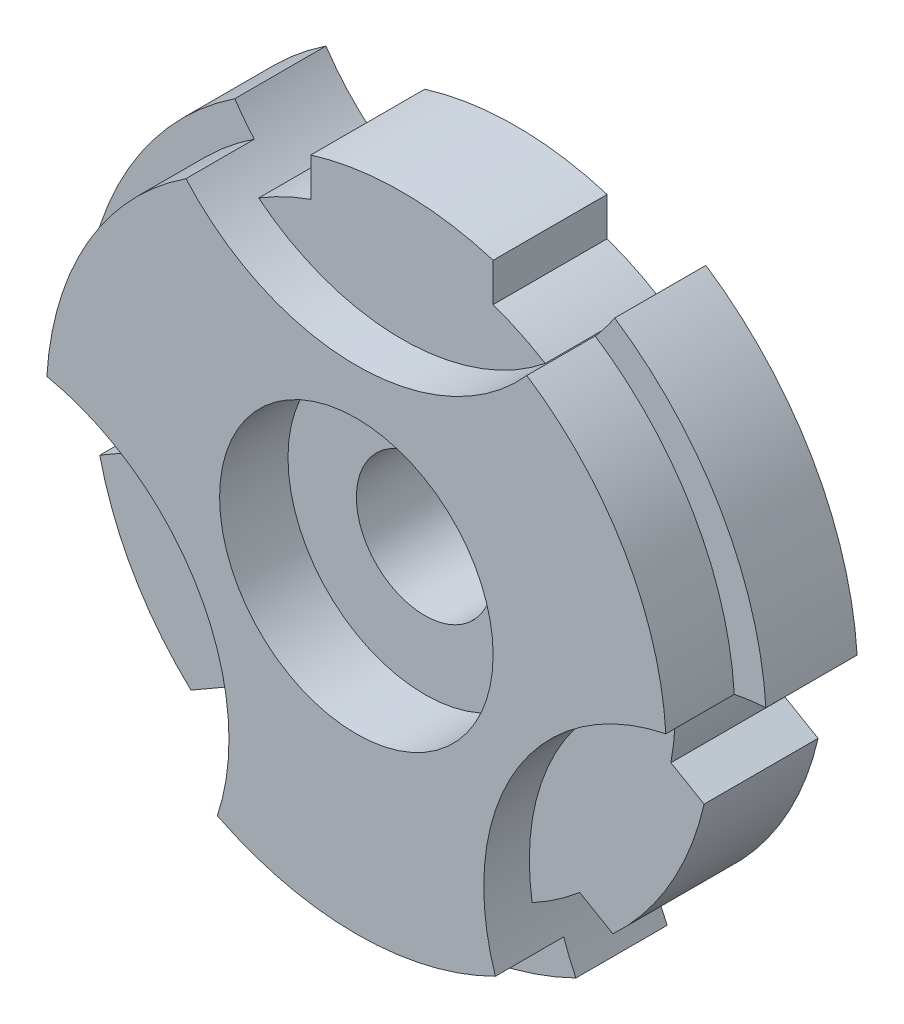
ISO-10303-21;
HEADER;
FILE_DESCRIPTION(('STEP AP214'),'2;1');
FILE_NAME('part.step','',(''),(''),'','','');
FILE_SCHEMA(('AUTOMOTIVE_DESIGN { 1 0 10303 214 1 1 1 1 }'));
ENDSEC;
DATA;
#1=APPLICATION_CONTEXT('core data for automotive mechanical design processes');
#2=APPLICATION_PROTOCOL_DEFINITION('international standard','automotive_design',2000,#1);
#3=PRODUCT_CONTEXT('',#1,'mechanical');
#4=PRODUCT('Part','Part','',(#3));
#5=PRODUCT_RELATED_PRODUCT_CATEGORY('part','',(#4));
#6=PRODUCT_DEFINITION_FORMATION('','',#4);
#7=PRODUCT_DEFINITION_CONTEXT('part definition',#1,'design');
#8=PRODUCT_DEFINITION('design','',#6,#7);
#9=PRODUCT_DEFINITION_SHAPE('','',#8);
#10=(LENGTH_UNIT() NAMED_UNIT(*) SI_UNIT(.MILLI.,.METRE.));
#11=(NAMED_UNIT(*) PLANE_ANGLE_UNIT() SI_UNIT($,.RADIAN.));
#12=(NAMED_UNIT(*) SI_UNIT($,.STERADIAN.) SOLID_ANGLE_UNIT());
#13=UNCERTAINTY_MEASURE_WITH_UNIT(LENGTH_MEASURE(1.E-05),#10,'distance_accuracy_value','');
#14=(GEOMETRIC_REPRESENTATION_CONTEXT(3) GLOBAL_UNCERTAINTY_ASSIGNED_CONTEXT((#13)) GLOBAL_UNIT_ASSIGNED_CONTEXT((#10,
#11,#12)) REPRESENTATION_CONTEXT('',''));
#15=CARTESIAN_POINT('',(0.,0.,0.));
#16=DIRECTION('',(0.,0.,1.));
#17=DIRECTION('',(1.,0.,0.));
#18=AXIS2_PLACEMENT_3D('',#15,#16,#17);
#19=CARTESIAN_POINT('',(0.,0.,20.));
#20=DIRECTION('',(0.,0.,-1.));
#21=DIRECTION('',(-1.,0.,0.));
#22=AXIS2_PLACEMENT_3D('',#19,#20,#21);
#23=CYLINDRICAL_SURFACE('',#22,75.);
#24=CARTESIAN_POINT('',(0.,0.,0.));
#25=DIRECTION('',(0.,0.,1.));
#26=DIRECTION('',(1.,0.,0.));
#27=AXIS2_PLACEMENT_3D('',#24,#25,#26);
#28=CIRCLE('',#27,75.);
#29=CARTESIAN_POINT('',(74.8395240227173,4.90363579939592,0.));
#30=VERTEX_POINT('',#29);
#31=CARTESIAN_POINT('',(41.6664351845422,62.3611111111111,0.));
#32=VERTEX_POINT('',#31);
#33=EDGE_CURVE('E459',#30,#32,#28,.T.);
#34=ORIENTED_EDGE('',*,*,#33,.T.);
#35=DIRECTION('',(0.,0.,1.));
#36=VECTOR('',#35,1.);
#37=CARTESIAN_POINT('',(41.6664351845422,62.3611111111111,17.5));
#38=LINE('',#37,#36);
#39=CARTESIAN_POINT('',(41.6664351845422,62.3611111111111,20.));
#40=VERTEX_POINT('',#39);
#41=EDGE_CURVE('E438',#32,#40,#38,.T.);
#42=ORIENTED_EDGE('',*,*,#41,.T.);
#43=CARTESIAN_POINT('',(0.,0.,20.));
#44=DIRECTION('',(0.,0.,1.));
#45=DIRECTION('',(1.,0.,0.));
#46=AXIS2_PLACEMENT_3D('',#43,#44,#45);
#47=CIRCLE('',#46,75.);
#48=CARTESIAN_POINT('',(74.8395240227173,4.90363579939591,20.));
#49=VERTEX_POINT('',#48);
#50=EDGE_CURVE('E455',#49,#40,#47,.T.);
#51=ORIENTED_EDGE('',*,*,#50,.F.);
#52=DIRECTION('',(0.,0.,1.));
#53=VECTOR('',#52,1.);
#54=CARTESIAN_POINT('',(74.8395240227173,4.90363579939593,17.5));
#55=LINE('',#54,#53);
#56=EDGE_CURVE('E417',#49,#30,#55,.F.);
#57=ORIENTED_EDGE('',*,*,#56,.T.);
#58=EDGE_LOOP('',(#34,#42,#51,#57));
#59=FACE_BOUND('',#58,.T.);
#60=ADVANCED_FACE('F50',(#59),#23,.T.);
#61=CARTESIAN_POINT('',(-33.1730888381753,-67.2647469105068,0.));
#62=VERTEX_POINT('',#61);
#63=CARTESIAN_POINT('',(33.1730888381754,-67.2647469105067,0.));
#64=VERTEX_POINT('',#63);
#65=EDGE_CURVE('E446',#62,#64,#28,.T.);
#66=ORIENTED_EDGE('',*,*,#65,.T.);
#67=DIRECTION('',(0.,0.,1.));
#68=VECTOR('',#67,1.);
#69=CARTESIAN_POINT('',(33.1730888381754,-67.2647469105067,17.5));
#70=LINE('',#69,#68);
#71=CARTESIAN_POINT('',(33.1730888381754,-67.2647469105067,20.));
#72=VERTEX_POINT('',#71);
#73=EDGE_CURVE('E424',#64,#72,#70,.T.);
#74=ORIENTED_EDGE('',*,*,#73,.T.);
#75=CARTESIAN_POINT('',(-33.1730888381753,-67.2647469105068,20.));
#76=VERTEX_POINT('',#75);
#77=EDGE_CURVE('E456',#76,#72,#47,.T.);
#78=ORIENTED_EDGE('',*,*,#77,.F.);
#79=DIRECTION('',(0.,0.,1.));
#80=VECTOR('',#79,1.);
#81=CARTESIAN_POINT('',(-33.1730888381753,-67.2647469105068,17.5));
#82=LINE('',#81,#80);
#83=EDGE_CURVE('E405',#76,#62,#82,.F.);
#84=ORIENTED_EDGE('',*,*,#83,.T.);
#85=EDGE_LOOP('',(#66,#74,#78,#84));
#86=FACE_BOUND('',#85,.T.);
#87=ADVANCED_FACE('F498',(#86),#23,.T.);
#88=CARTESIAN_POINT('',(0.,0.,20.));
#89=DIRECTION('',(0.,0.,1.));
#90=DIRECTION('',(1.,0.,0.));
#91=AXIS2_PLACEMENT_3D('',#88,#89,#90);
#92=PLANE('',#91);
#93=CARTESIAN_POINT('',(0.,90.,20.));
#94=DIRECTION('',(0.,0.,1.));
#95=DIRECTION('',(1.,0.,0.));
#96=AXIS2_PLACEMENT_3D('',#93,#94,#95);
#97=CIRCLE('',#96,50.);
#98=CARTESIAN_POINT('',(-41.6664351845422,62.3611111111111,20.));
#99=VERTEX_POINT('',#98);
#100=CARTESIAN_POINT('',(-37.3866286257534,56.8,20.));
#101=VERTEX_POINT('',#100);
#102=EDGE_CURVE('E429',#99,#101,#97,.T.);
#103=ORIENTED_EDGE('',*,*,#102,.F.);
#104=CARTESIAN_POINT('',(-74.8395240227173,4.90363579939591,20.));
#105=VERTEX_POINT('',#104);
#106=EDGE_CURVE('E460',#99,#105,#47,.T.);
#107=ORIENTED_EDGE('',*,*,#106,.T.);
#108=CARTESIAN_POINT('',(-77.9422863405996,-44.9999999999998,20.));
#109=DIRECTION('',(0.,0.,1.));
#110=DIRECTION('',(1.,0.,0.));
#111=AXIS2_PLACEMENT_3D('',#108,#109,#110);
#112=CIRCLE('',#111,50.);
#113=CARTESIAN_POINT('',(-67.8835572478328,3.97777015175706,20.));
#114=VERTEX_POINT('',#113);
#115=EDGE_CURVE('E401',#114,#105,#112,.T.);
#116=ORIENTED_EDGE('',*,*,#115,.F.);
#117=CARTESIAN_POINT('',(0.,0.,20.));
#118=DIRECTION('',(0.,0.,1.));
#119=DIRECTION('',(1.,0.,0.));
#120=AXIS2_PLACEMENT_3D('',#117,#118,#119);
#121=CIRCLE('',#120,68.);
#122=EDGE_CURVE('E454',#101,#114,#121,.T.);
#123=ORIENTED_EDGE('',*,*,#122,.F.);
#124=EDGE_LOOP('',(#103,#107,#116,#123));
#125=FACE_BOUND('',#124,.T.);
#126=ADVANCED_FACE('F489',(#125),#92,.T.);
#127=CARTESIAN_POINT('',(37.3866286257534,56.8,20.));
#128=VERTEX_POINT('',#127);
#129=EDGE_CURVE('E433',#128,#40,#97,.T.);
#130=ORIENTED_EDGE('',*,*,#129,.F.);
#131=CARTESIAN_POINT('',(67.8835572478328,3.97777015175707,20.));
#132=VERTEX_POINT('',#131);
#133=EDGE_CURVE('E449',#132,#128,#121,.T.);
#134=ORIENTED_EDGE('',*,*,#133,.F.);
#135=CARTESIAN_POINT('',(77.9422863405996,-44.9999999999998,20.));
#136=DIRECTION('',(0.,0.,1.));
#137=DIRECTION('',(1.,0.,0.));
#138=AXIS2_PLACEMENT_3D('',#135,#136,#137);
#139=CIRCLE('',#138,50.);
#140=EDGE_CURVE('E411',#49,#132,#139,.T.);
#141=ORIENTED_EDGE('',*,*,#140,.F.);
#142=ORIENTED_EDGE('',*,*,#50,.T.);
#143=EDGE_LOOP('',(#130,#134,#141,#142));
#144=FACE_BOUND('',#143,.T.);
#145=ADVANCED_FACE('F542',(#144),#92,.T.);
#146=CARTESIAN_POINT('',(0.,0.,35.));
#147=DIRECTION('',(0.,0.,-1.));
#148=DIRECTION('',(-1.,0.,0.));
#149=AXIS2_PLACEMENT_3D('',#146,#147,#148);
#150=CYLINDRICAL_SURFACE('',#149,68.);
#151=ORIENTED_EDGE('',*,*,#133,.T.);
#152=DIRECTION('',(0.,0.,1.));
#153=VECTOR('',#152,1.);
#154=CARTESIAN_POINT('',(37.3866286257534,56.8,17.5));
#155=LINE('',#154,#153);
#156=CARTESIAN_POINT('',(37.3866286257534,56.8,35.));
#157=VERTEX_POINT('',#156);
#158=EDGE_CURVE('E436',#128,#157,#155,.T.);
#159=ORIENTED_EDGE('',*,*,#158,.T.);
#160=CARTESIAN_POINT('',(0.,0.,35.));
#161=DIRECTION('',(0.,0.,1.));
#162=DIRECTION('',(1.,0.,0.));
#163=AXIS2_PLACEMENT_3D('',#160,#161,#162);
#164=CIRCLE('',#163,68.);
#165=CARTESIAN_POINT('',(67.8835572478328,3.97777015175707,35.));
#166=VERTEX_POINT('',#165);
#167=EDGE_CURVE('E444',#166,#157,#164,.T.);
#168=ORIENTED_EDGE('',*,*,#167,.F.);
#169=DIRECTION('',(0.,0.,1.));
#170=VECTOR('',#169,1.);
#171=CARTESIAN_POINT('',(67.8835572478328,3.97777015175708,17.5));
#172=LINE('',#171,#170);
#173=EDGE_CURVE('E414',#166,#132,#172,.F.);
#174=ORIENTED_EDGE('',*,*,#173,.T.);
#175=EDGE_LOOP('',(#151,#159,#168,#174));
#176=FACE_BOUND('',#175,.T.);
#177=ADVANCED_FACE('F546',(#176),#150,.T.);
#178=CARTESIAN_POINT('',(-30.4969286220795,-60.7777701517569,20.));
#179=VERTEX_POINT('',#178);
#180=CARTESIAN_POINT('',(30.4969286220796,-60.7777701517568,20.));
#181=VERTEX_POINT('',#180);
#182=EDGE_CURVE('E452',#179,#181,#121,.T.);
#183=ORIENTED_EDGE('',*,*,#182,.T.);
#184=DIRECTION('',(0.,0.,1.));
#185=VECTOR('',#184,1.);
#186=CARTESIAN_POINT('',(30.4969286220796,-60.7777701517568,17.5));
#187=LINE('',#186,#185);
#188=CARTESIAN_POINT('',(30.4969286220796,-60.7777701517568,35.));
#189=VERTEX_POINT('',#188);
#190=EDGE_CURVE('E423',#181,#189,#187,.T.);
#191=ORIENTED_EDGE('',*,*,#190,.T.);
#192=CARTESIAN_POINT('',(-30.4969286220796,-60.7777701517568,35.));
#193=VERTEX_POINT('',#192);
#194=EDGE_CURVE('E445',#193,#189,#164,.T.);
#195=ORIENTED_EDGE('',*,*,#194,.F.);
#196=DIRECTION('',(0.,0.,1.));
#197=VECTOR('',#196,1.);
#198=CARTESIAN_POINT('',(-30.4969286220796,-60.7777701517568,17.5));
#199=LINE('',#198,#197);
#200=EDGE_CURVE('E388',#193,#179,#199,.F.);
#201=ORIENTED_EDGE('',*,*,#200,.T.);
#202=EDGE_LOOP('',(#183,#191,#195,#201));
#203=FACE_BOUND('',#202,.T.);
#204=ADVANCED_FACE('F475',(#203),#150,.T.);
#205=ORIENTED_EDGE('',*,*,#106,.F.);
#206=DIRECTION('',(0.,0.,1.));
#207=VECTOR('',#206,1.);
#208=CARTESIAN_POINT('',(-41.6664351845422,62.3611111111111,17.5));
#209=LINE('',#208,#207);
#210=CARTESIAN_POINT('',(-41.6664351845422,62.3611111111111,0.));
#211=VERTEX_POINT('',#210);
#212=EDGE_CURVE('E435',#99,#211,#209,.F.);
#213=ORIENTED_EDGE('',*,*,#212,.T.);
#214=CARTESIAN_POINT('',(-74.8395240227173,4.9036357993959,0.));
#215=VERTEX_POINT('',#214);
#216=EDGE_CURVE('E462',#211,#215,#28,.T.);
#217=ORIENTED_EDGE('',*,*,#216,.T.);
#218=DIRECTION('',(0.,0.,1.));
#219=VECTOR('',#218,1.);
#220=CARTESIAN_POINT('',(-74.8395240227173,4.9036357993959,17.5));
#221=LINE('',#220,#219);
#222=EDGE_CURVE('E408',#215,#105,#221,.T.);
#223=ORIENTED_EDGE('',*,*,#222,.T.);
#224=EDGE_LOOP('',(#205,#213,#217,#223));
#225=FACE_BOUND('',#224,.T.);
#226=ADVANCED_FACE('F47',(#225),#23,.T.);
#227=EDGE_CURVE('E416',#181,#72,#139,.T.);
#228=ORIENTED_EDGE('',*,*,#227,.F.);
#229=ORIENTED_EDGE('',*,*,#182,.F.);
#230=EDGE_CURVE('E396',#76,#179,#112,.T.);
#231=ORIENTED_EDGE('',*,*,#230,.F.);
#232=ORIENTED_EDGE('',*,*,#77,.T.);
#233=EDGE_LOOP('',(#228,#229,#231,#232));
#234=FACE_BOUND('',#233,.T.);
#235=ADVANCED_FACE('F500',(#234),#92,.T.);
#236=CARTESIAN_POINT('',(0.,0.,0.));
#237=DIRECTION('',(0.,0.,1.));
#238=DIRECTION('',(1.,0.,0.));
#239=AXIS2_PLACEMENT_3D('',#236,#237,#238);
#240=PLANE('',#239);
#241=CARTESIAN_POINT('',(0.,0.,0.));
#242=DIRECTION('',(0.,0.,1.));
#243=DIRECTION('',(1.,0.,0.));
#244=AXIS2_PLACEMENT_3D('',#241,#242,#243);
#245=CIRCLE('',#244,15.);
#246=CARTESIAN_POINT('',(15.,0.,0.));
#247=VERTEX_POINT('',#246);
#248=EDGE_CURVE('E1009',#247,#247,#245,.T.);
#249=ORIENTED_EDGE('',*,*,#248,.T.);
#250=EDGE_LOOP('',(#249));
#251=FACE_BOUND('',#250,.T.);
#252=ORIENTED_EDGE('',*,*,#216,.F.);
#253=CARTESIAN_POINT('',(0.,90.,0.));
#254=DIRECTION('',(0.,0.,1.));
#255=DIRECTION('',(1.,0.,0.));
#256=AXIS2_PLACEMENT_3D('',#253,#254,#255);
#257=CIRCLE('',#256,50.);
#258=CARTESIAN_POINT('',(-31.4269680527354,51.1111111111111,0.));
#259=VERTEX_POINT('',#258);
#260=EDGE_CURVE('E390',#211,#259,#257,.T.);
#261=ORIENTED_EDGE('',*,*,#260,.T.);
#262=CARTESIAN_POINT('',(0.,0.,0.));
#263=DIRECTION('',(0.,0.,-1.));
#264=DIRECTION('',(-1.,0.,0.));
#265=AXIS2_PLACEMENT_3D('',#262,#263,#264);
#266=CIRCLE('',#265,60.);
#267=CARTESIAN_POINT('',(-20.0000000000003,56.5685424949237,0.));
#268=VERTEX_POINT('',#267);
#269=EDGE_CURVE('E364',#259,#268,#266,.T.);
#270=ORIENTED_EDGE('',*,*,#269,.T.);
#271=DIRECTION('',(0.,-1.,0.));
#272=VECTOR('',#271,1.);
#273=CARTESIAN_POINT('',(-20.0000000000003,0.,0.));
#274=LINE('',#273,#272);
#275=CARTESIAN_POINT('',(-20.0000000000003,64.9923072370876,0.));
#276=VERTEX_POINT('',#275);
#277=EDGE_CURVE('E366',#276,#268,#274,.T.);
#278=ORIENTED_EDGE('',*,*,#277,.F.);
#279=CARTESIAN_POINT('',(0.,0.,0.));
#280=DIRECTION('',(0.,0.,-1.));
#281=DIRECTION('',(-1.,0.,0.));
#282=AXIS2_PLACEMENT_3D('',#279,#280,#281);
#283=CIRCLE('',#282,68.);
#284=CARTESIAN_POINT('',(20.0000000000015,64.9923072370872,0.));
#285=VERTEX_POINT('',#284);
#286=EDGE_CURVE('E350',#276,#285,#283,.T.);
#287=ORIENTED_EDGE('',*,*,#286,.T.);
#288=DIRECTION('',(0.,1.,0.));
#289=VECTOR('',#288,1.);
#290=CARTESIAN_POINT('',(20.0000000000016,0.,0.));
#291=LINE('',#290,#289);
#292=CARTESIAN_POINT('',(20.0000000000015,56.5685424949233,0.));
#293=VERTEX_POINT('',#292);
#294=EDGE_CURVE('E334',#293,#285,#291,.T.);
#295=ORIENTED_EDGE('',*,*,#294,.F.);
#296=CARTESIAN_POINT('',(0.,0.,0.));
#297=DIRECTION('',(0.,0.,-1.));
#298=DIRECTION('',(-1.,0.,0.));
#299=AXIS2_PLACEMENT_3D('',#296,#297,#298);
#300=CIRCLE('',#299,60.);
#301=CARTESIAN_POINT('',(31.4269680527354,51.1111111111111,0.));
#302=VERTEX_POINT('',#301);
#303=EDGE_CURVE('E361',#293,#302,#300,.T.);
#304=ORIENTED_EDGE('',*,*,#303,.T.);
#305=EDGE_CURVE('E391',#302,#32,#257,.T.);
#306=ORIENTED_EDGE('',*,*,#305,.T.);
#307=ORIENTED_EDGE('',*,*,#33,.F.);
#308=CARTESIAN_POINT('',(77.9422863405996,-44.9999999999998,0.));
#309=DIRECTION('',(0.,0.,1.));
#310=DIRECTION('',(1.,0.,0.));
#311=AXIS2_PLACEMENT_3D('',#308,#309,#310);
#312=CIRCLE('',#311,50.);
#313=CARTESIAN_POINT('',(59.977004664239,1.66099714203546,0.));
#314=VERTEX_POINT('',#313);
#315=EDGE_CURVE('E392',#30,#314,#312,.T.);
#316=ORIENTED_EDGE('',*,*,#315,.T.);
#317=CARTESIAN_POINT('',(0.,0.,0.));
#318=DIRECTION('',(0.,0.,-1.));
#319=DIRECTION('',(-1.,0.,0.));
#320=AXIS2_PLACEMENT_3D('',#317,#318,#319);
#321=CIRCLE('',#320,60.);
#322=CARTESIAN_POINT('',(58.9897948556636,-10.9637631717728,0.));
#323=VERTEX_POINT('',#322);
#324=EDGE_CURVE('E293',#314,#323,#321,.T.);
#325=ORIENTED_EDGE('',*,*,#324,.T.);
#326=DIRECTION('',(-0.866025403784439,0.5,0.));
#327=VECTOR('',#326,1.);
#328=CARTESIAN_POINT('',(10.0000000000001,17.320508075689,0.));
#329=LINE('',#328,#327);
#330=CARTESIAN_POINT('',(66.2849891178813,-15.1756455428548,0.));
#331=VERTEX_POINT('',#330);
#332=EDGE_CURVE('E321',#331,#323,#329,.T.);
#333=ORIENTED_EDGE('',*,*,#332,.F.);
#334=CARTESIAN_POINT('',(0.,0.,0.));
#335=DIRECTION('',(0.,0.,-1.));
#336=DIRECTION('',(-1.,0.,0.));
#337=AXIS2_PLACEMENT_3D('',#334,#335,#336);
#338=CIRCLE('',#337,68.);
#339=CARTESIAN_POINT('',(46.28498911788,-49.8166616942337,0.));
#340=VERTEX_POINT('',#339);
#341=EDGE_CURVE('E322',#331,#340,#338,.T.);
#342=ORIENTED_EDGE('',*,*,#341,.T.);
#343=DIRECTION('',(0.866025403784439,-0.5,0.));
#344=VECTOR('',#343,1.);
#345=CARTESIAN_POINT('',(-10.0000000000008,-17.3205080756901,0.));
#346=LINE('',#345,#344);
#347=CARTESIAN_POINT('',(38.9897948556623,-45.6047793231517,0.));
#348=VERTEX_POINT('',#347);
#349=EDGE_CURVE('E330',#348,#340,#346,.T.);
#350=ORIENTED_EDGE('',*,*,#349,.F.);
#351=CARTESIAN_POINT('',(0.,0.,0.));
#352=DIRECTION('',(0.,0.,-1.));
#353=DIRECTION('',(-1.,0.,0.));
#354=AXIS2_PLACEMENT_3D('',#351,#352,#353);
#355=CIRCLE('',#354,60.);
#356=CARTESIAN_POINT('',(28.5500366115038,-52.7721082531463,0.));
#357=VERTEX_POINT('',#356);
#358=EDGE_CURVE('E70',#348,#357,#355,.T.);
#359=ORIENTED_EDGE('',*,*,#358,.T.);
#360=EDGE_CURVE('E395',#357,#64,#312,.T.);
#361=ORIENTED_EDGE('',*,*,#360,.T.);
#362=ORIENTED_EDGE('',*,*,#65,.F.);
#363=CARTESIAN_POINT('',(-77.9422863405996,-44.9999999999998,0.));
#364=DIRECTION('',(0.,0.,1.));
#365=DIRECTION('',(1.,0.,0.));
#366=AXIS2_PLACEMENT_3D('',#363,#364,#365);
#367=CIRCLE('',#366,50.);
#368=CARTESIAN_POINT('',(-28.5500366115037,-52.7721082531464,0.));
#369=VERTEX_POINT('',#368);
#370=EDGE_CURVE('E398',#62,#369,#367,.T.);
#371=ORIENTED_EDGE('',*,*,#370,.T.);
#372=CARTESIAN_POINT('',(0.,0.,0.));
#373=DIRECTION('',(0.,0.,-1.));
#374=DIRECTION('',(-1.,0.,0.));
#375=AXIS2_PLACEMENT_3D('',#372,#373,#374);
#376=CIRCLE('',#375,60.);
#377=CARTESIAN_POINT('',(-38.9897948556636,-45.6047793231507,0.));
#378=VERTEX_POINT('',#377);
#379=EDGE_CURVE('E250',#369,#378,#376,.T.);
#380=ORIENTED_EDGE('',*,*,#379,.T.);
#381=DIRECTION('',(0.866025403784418,0.500000000000035,0.));
#382=VECTOR('',#381,1.);
#383=CARTESIAN_POINT('',(9.99999999999954,-17.3205080756863,0.));
#384=LINE('',#383,#382);
#385=CARTESIAN_POINT('',(-46.2849891178809,-49.8166616942328,0.));
#386=VERTEX_POINT('',#385);
#387=EDGE_CURVE('E285',#386,#378,#384,.T.);
#388=ORIENTED_EDGE('',*,*,#387,.F.);
#389=CARTESIAN_POINT('',(0.,0.,0.));
#390=DIRECTION('',(0.,0.,-1.));
#391=DIRECTION('',(-1.,0.,0.));
#392=AXIS2_PLACEMENT_3D('',#389,#390,#391);
#393=CIRCLE('',#392,68.);
#394=CARTESIAN_POINT('',(-66.2849891178815,-15.1756455428535,0.));
#395=VERTEX_POINT('',#394);
#396=EDGE_CURVE('E290',#386,#395,#393,.T.);
#397=ORIENTED_EDGE('',*,*,#396,.T.);
#398=DIRECTION('',(-0.866025403784439,-0.5,0.));
#399=VECTOR('',#398,1.);
#400=CARTESIAN_POINT('',(-10.0000000000008,17.3205080756901,0.));
#401=LINE('',#400,#399);
#402=CARTESIAN_POINT('',(-58.9897948556639,-10.9637631717715,0.));
#403=VERTEX_POINT('',#402);
#404=EDGE_CURVE('E271',#403,#395,#401,.T.);
#405=ORIENTED_EDGE('',*,*,#404,.F.);
#406=CARTESIAN_POINT('',(0.,0.,0.));
#407=DIRECTION('',(0.,0.,-1.));
#408=DIRECTION('',(-1.,0.,0.));
#409=AXIS2_PLACEMENT_3D('',#406,#407,#408);
#410=CIRCLE('',#409,60.);
#411=CARTESIAN_POINT('',(-59.977004664239,1.66099714203546,0.));
#412=VERTEX_POINT('',#411);
#413=EDGE_CURVE('E62',#403,#412,#410,.T.);
#414=ORIENTED_EDGE('',*,*,#413,.T.);
#415=EDGE_CURVE('E374',#412,#215,#367,.T.);
#416=ORIENTED_EDGE('',*,*,#415,.T.);
#417=EDGE_LOOP('',(#252,#261,#270,#278,#287,#295,#304,#306,#307,#316,#325,#333,#342,#350,#359,
#361,#362,#371,#380,#388,#397,#405,#414,#416));
#418=FACE_BOUND('',#417,.T.);
#419=ADVANCED_FACE('F508',(#251,#418),#240,.F.);
#420=CARTESIAN_POINT('',(-37.3866286257534,56.8,35.));
#421=VERTEX_POINT('',#420);
#422=CARTESIAN_POINT('',(-67.8835572478328,3.97777015175706,35.));
#423=VERTEX_POINT('',#422);
#424=EDGE_CURVE('E447',#421,#423,#164,.T.);
#425=ORIENTED_EDGE('',*,*,#424,.F.);
#426=DIRECTION('',(0.,0.,1.));
#427=VECTOR('',#426,1.);
#428=CARTESIAN_POINT('',(-37.3866286257534,56.8,17.5));
#429=LINE('',#428,#427);
#430=EDGE_CURVE('E430',#421,#101,#429,.F.);
#431=ORIENTED_EDGE('',*,*,#430,.T.);
#432=ORIENTED_EDGE('',*,*,#122,.T.);
#433=DIRECTION('',(0.,0.,1.));
#434=VECTOR('',#433,1.);
#435=CARTESIAN_POINT('',(-67.8835572478328,3.97777015175706,17.5));
#436=LINE('',#435,#434);
#437=EDGE_CURVE('E406',#114,#423,#436,.T.);
#438=ORIENTED_EDGE('',*,*,#437,.T.);
#439=EDGE_LOOP('',(#425,#431,#432,#438));
#440=FACE_BOUND('',#439,.T.);
#441=ADVANCED_FACE('F485',(#440),#150,.T.);
#442=CARTESIAN_POINT('',(0.,0.,35.));
#443=DIRECTION('',(0.,0.,1.));
#444=DIRECTION('',(1.,0.,0.));
#445=AXIS2_PLACEMENT_3D('',#442,#443,#444);
#446=PLANE('',#445);
#447=CARTESIAN_POINT('',(0.,0.,35.));
#448=DIRECTION('',(0.,0.,1.));
#449=DIRECTION('',(1.,0.,0.));
#450=AXIS2_PLACEMENT_3D('',#447,#448,#449);
#451=CIRCLE('',#450,30.);
#452=CARTESIAN_POINT('',(30.,0.,35.));
#453=VERTEX_POINT('',#452);
#454=EDGE_CURVE('E273',#453,#453,#451,.T.);
#455=ORIENTED_EDGE('',*,*,#454,.F.);
#456=EDGE_LOOP('',(#455));
#457=FACE_BOUND('',#456,.T.);
#458=CARTESIAN_POINT('',(0.,90.,35.));
#459=DIRECTION('',(0.,0.,1.));
#460=DIRECTION('',(1.,0.,0.));
#461=AXIS2_PLACEMENT_3D('',#458,#459,#460);
#462=CIRCLE('',#461,50.);
#463=EDGE_CURVE('E11',#421,#157,#462,.T.);
#464=ORIENTED_EDGE('',*,*,#463,.F.);
#465=ORIENTED_EDGE('',*,*,#424,.T.);
#466=CARTESIAN_POINT('',(-77.9422863405996,-44.9999999999998,35.));
#467=DIRECTION('',(0.,0.,1.));
#468=DIRECTION('',(1.,0.,0.));
#469=AXIS2_PLACEMENT_3D('',#466,#467,#468);
#470=CIRCLE('',#469,50.);
#471=EDGE_CURVE('E453',#193,#423,#470,.T.);
#472=ORIENTED_EDGE('',*,*,#471,.F.);
#473=ORIENTED_EDGE('',*,*,#194,.T.);
#474=CARTESIAN_POINT('',(77.9422863405996,-44.9999999999998,35.));
#475=DIRECTION('',(0.,0.,1.));
#476=DIRECTION('',(1.,0.,0.));
#477=AXIS2_PLACEMENT_3D('',#474,#475,#476);
#478=CIRCLE('',#477,50.);
#479=EDGE_CURVE('E54',#166,#189,#478,.T.);
#480=ORIENTED_EDGE('',*,*,#479,.F.);
#481=ORIENTED_EDGE('',*,*,#167,.T.);
#482=EDGE_LOOP('',(#464,#465,#472,#473,#480,#481));
#483=FACE_BOUND('',#482,.T.);
#484=ADVANCED_FACE('F476',(#457,#483),#446,.T.);
#485=CARTESIAN_POINT('',(-77.9422863405996,-44.9999999999998,0.));
#486=DIRECTION('',(0.,0.,1.));
#487=DIRECTION('',(1.,0.,0.));
#488=AXIS2_PLACEMENT_3D('',#485,#486,#487);
#489=CYLINDRICAL_SURFACE('',#488,50.);
#490=ORIENTED_EDGE('',*,*,#415,.F.);
#491=DIRECTION('',(0.,0.,-1.));
#492=VECTOR('',#491,1.);
#493=CARTESIAN_POINT('',(-59.977004664239,1.66099714203546,25.));
#494=LINE('',#493,#492);
#495=CARTESIAN_POINT('',(-59.977004664239,1.66099714203546,25.));
#496=VERTEX_POINT('',#495);
#497=EDGE_CURVE('E267',#496,#412,#494,.T.);
#498=ORIENTED_EDGE('',*,*,#497,.F.);
#499=CARTESIAN_POINT('',(-77.9422863405996,-44.9999999999998,25.));
#500=DIRECTION('',(0.,0.,-1.));
#501=DIRECTION('',(-1.,0.,0.));
#502=AXIS2_PLACEMENT_3D('',#499,#500,#501);
#503=CIRCLE('',#502,50.);
#504=CARTESIAN_POINT('',(-28.5500366115037,-52.7721082531464,25.));
#505=VERTEX_POINT('',#504);
#506=EDGE_CURVE('E259',#505,#496,#503,.F.);
#507=ORIENTED_EDGE('',*,*,#506,.F.);
#508=DIRECTION('',(0.,0.,-1.));
#509=VECTOR('',#508,1.);
#510=CARTESIAN_POINT('',(-28.5500366115037,-52.7721082531464,25.));
#511=LINE('',#510,#509);
#512=EDGE_CURVE('E243',#505,#369,#511,.T.);
#513=ORIENTED_EDGE('',*,*,#512,.T.);
#514=ORIENTED_EDGE('',*,*,#370,.F.);
#515=ORIENTED_EDGE('',*,*,#83,.F.);
#516=ORIENTED_EDGE('',*,*,#230,.T.);
#517=ORIENTED_EDGE('',*,*,#200,.F.);
#518=ORIENTED_EDGE('',*,*,#471,.T.);
#519=ORIENTED_EDGE('',*,*,#437,.F.);
#520=ORIENTED_EDGE('',*,*,#115,.T.);
#521=ORIENTED_EDGE('',*,*,#222,.F.);
#522=EDGE_LOOP('',(#490,#498,#507,#513,#514,#515,#516,#517,#518,#519,#520,#521));
#523=FACE_BOUND('',#522,.T.);
#524=ADVANCED_FACE('F268',(#523),#489,.F.);
#525=CARTESIAN_POINT('',(77.9422863405996,-44.9999999999998,0.));
#526=DIRECTION('',(0.,0.,1.));
#527=DIRECTION('',(1.,0.,0.));
#528=AXIS2_PLACEMENT_3D('',#525,#526,#527);
#529=CYLINDRICAL_SURFACE('',#528,50.);
#530=ORIENTED_EDGE('',*,*,#360,.F.);
#531=DIRECTION('',(0.,0.,-1.));
#532=VECTOR('',#531,1.);
#533=CARTESIAN_POINT('',(28.5500366115038,-52.7721082531463,25.));
#534=LINE('',#533,#532);
#535=CARTESIAN_POINT('',(28.5500366115038,-52.7721082531463,25.));
#536=VERTEX_POINT('',#535);
#537=EDGE_CURVE('E332',#536,#357,#534,.T.);
#538=ORIENTED_EDGE('',*,*,#537,.F.);
#539=CARTESIAN_POINT('',(77.9422863405996,-44.9999999999998,25.));
#540=DIRECTION('',(0.,0.,-1.));
#541=DIRECTION('',(-1.,0.,0.));
#542=AXIS2_PLACEMENT_3D('',#539,#540,#541);
#543=CIRCLE('',#542,50.);
#544=CARTESIAN_POINT('',(59.977004664239,1.66099714203546,25.));
#545=VERTEX_POINT('',#544);
#546=EDGE_CURVE('E302',#545,#536,#543,.F.);
#547=ORIENTED_EDGE('',*,*,#546,.F.);
#548=DIRECTION('',(0.,0.,-1.));
#549=VECTOR('',#548,1.);
#550=CARTESIAN_POINT('',(59.977004664239,1.66099714203546,25.));
#551=LINE('',#550,#549);
#552=EDGE_CURVE('E318',#545,#314,#551,.T.);
#553=ORIENTED_EDGE('',*,*,#552,.T.);
#554=ORIENTED_EDGE('',*,*,#315,.F.);
#555=ORIENTED_EDGE('',*,*,#56,.F.);
#556=ORIENTED_EDGE('',*,*,#140,.T.);
#557=ORIENTED_EDGE('',*,*,#173,.F.);
#558=ORIENTED_EDGE('',*,*,#479,.T.);
#559=ORIENTED_EDGE('',*,*,#190,.F.);
#560=ORIENTED_EDGE('',*,*,#227,.T.);
#561=ORIENTED_EDGE('',*,*,#73,.F.);
#562=EDGE_LOOP('',(#530,#538,#547,#553,#554,#555,#556,#557,#558,#559,#560,#561));
#563=FACE_BOUND('',#562,.T.);
#564=ADVANCED_FACE('F468',(#563),#529,.F.);
#565=CARTESIAN_POINT('',(0.,90.,0.));
#566=DIRECTION('',(0.,0.,1.));
#567=DIRECTION('',(1.,0.,0.));
#568=AXIS2_PLACEMENT_3D('',#565,#566,#567);
#569=CYLINDRICAL_SURFACE('',#568,50.);
#570=CARTESIAN_POINT('',(0.,90.,25.));
#571=DIRECTION('',(0.,0.,-1.));
#572=DIRECTION('',(-1.,0.,0.));
#573=AXIS2_PLACEMENT_3D('',#570,#571,#572);
#574=CIRCLE('',#573,50.);
#575=CARTESIAN_POINT('',(-31.4269680527354,51.1111111111111,25.));
#576=VERTEX_POINT('',#575);
#577=CARTESIAN_POINT('',(31.4269680527355,51.1111111111111,25.));
#578=VERTEX_POINT('',#577);
#579=EDGE_CURVE('E348',#576,#578,#574,.F.);
#580=ORIENTED_EDGE('',*,*,#579,.F.);
#581=DIRECTION('',(0.,0.,-1.));
#582=VECTOR('',#581,1.);
#583=CARTESIAN_POINT('',(-31.4269680527354,51.1111111111111,25.));
#584=LINE('',#583,#582);
#585=EDGE_CURVE('E379',#576,#259,#584,.T.);
#586=ORIENTED_EDGE('',*,*,#585,.T.);
#587=ORIENTED_EDGE('',*,*,#260,.F.);
#588=ORIENTED_EDGE('',*,*,#212,.F.);
#589=ORIENTED_EDGE('',*,*,#102,.T.);
#590=ORIENTED_EDGE('',*,*,#430,.F.);
#591=ORIENTED_EDGE('',*,*,#463,.T.);
#592=ORIENTED_EDGE('',*,*,#158,.F.);
#593=ORIENTED_EDGE('',*,*,#129,.T.);
#594=ORIENTED_EDGE('',*,*,#41,.F.);
#595=ORIENTED_EDGE('',*,*,#305,.F.);
#596=DIRECTION('',(0.,0.,-1.));
#597=VECTOR('',#596,1.);
#598=CARTESIAN_POINT('',(31.4269680527355,51.1111111111111,25.));
#599=LINE('',#598,#597);
#600=EDGE_CURVE('E382',#578,#302,#599,.T.);
#601=ORIENTED_EDGE('',*,*,#600,.F.);
#602=EDGE_LOOP('',(#580,#586,#587,#588,#589,#590,#591,#592,#593,#594,#595,#601));
#603=FACE_BOUND('',#602,.T.);
#604=ADVANCED_FACE('F512',(#603),#569,.F.);
#605=CARTESIAN_POINT('',(20.0000000000016,0.,25.));
#606=DIRECTION('',(-1.,0.,0.));
#607=DIRECTION('',(0.,-1.,0.));
#608=AXIS2_PLACEMENT_3D('',#605,#606,#607);
#609=PLANE('',#608);
#610=ORIENTED_EDGE('',*,*,#294,.T.);
#611=DIRECTION('',(0.,0.,-1.));
#612=VECTOR('',#611,1.);
#613=CARTESIAN_POINT('',(20.0000000000015,64.9923072370872,25.));
#614=LINE('',#613,#612);
#615=CARTESIAN_POINT('',(20.0000000000015,64.9923072370872,25.));
#616=VERTEX_POINT('',#615);
#617=EDGE_CURVE('E373',#616,#285,#614,.T.);
#618=ORIENTED_EDGE('',*,*,#617,.F.);
#619=DIRECTION('',(0.,1.,0.));
#620=VECTOR('',#619,1.);
#621=CARTESIAN_POINT('',(20.0000000000016,0.,25.));
#622=LINE('',#621,#620);
#623=CARTESIAN_POINT('',(20.0000000000015,56.5685424949233,25.));
#624=VERTEX_POINT('',#623);
#625=EDGE_CURVE('E345',#624,#616,#622,.T.);
#626=ORIENTED_EDGE('',*,*,#625,.F.);
#627=DIRECTION('',(0.,0.,-1.));
#628=VECTOR('',#627,1.);
#629=CARTESIAN_POINT('',(20.0000000000015,56.5685424949233,25.));
#630=LINE('',#629,#628);
#631=EDGE_CURVE('E356',#624,#293,#630,.T.);
#632=ORIENTED_EDGE('',*,*,#631,.T.);
#633=EDGE_LOOP('',(#610,#618,#626,#632));
#634=FACE_BOUND('',#633,.T.);
#635=ADVANCED_FACE('F533',(#634),#609,.F.);
#636=CARTESIAN_POINT('',(0.,0.,25.));
#637=DIRECTION('',(0.,0.,-1.));
#638=DIRECTION('',(-1.,0.,0.));
#639=AXIS2_PLACEMENT_3D('',#636,#637,#638);
#640=CYLINDRICAL_SURFACE('',#639,68.);
#641=ORIENTED_EDGE('',*,*,#286,.F.);
#642=DIRECTION('',(0.,0.,-1.));
#643=VECTOR('',#642,1.);
#644=CARTESIAN_POINT('',(-20.0000000000003,64.9923072370876,25.));
#645=LINE('',#644,#643);
#646=CARTESIAN_POINT('',(-20.0000000000003,64.9923072370876,25.));
#647=VERTEX_POINT('',#646);
#648=EDGE_CURVE('E376',#647,#276,#645,.T.);
#649=ORIENTED_EDGE('',*,*,#648,.F.);
#650=CARTESIAN_POINT('',(0.,0.,25.));
#651=DIRECTION('',(0.,0.,-1.));
#652=DIRECTION('',(-1.,0.,0.));
#653=AXIS2_PLACEMENT_3D('',#650,#651,#652);
#654=CIRCLE('',#653,68.);
#655=EDGE_CURVE('E359',#647,#616,#654,.T.);
#656=ORIENTED_EDGE('',*,*,#655,.T.);
#657=ORIENTED_EDGE('',*,*,#617,.T.);
#658=EDGE_LOOP('',(#641,#649,#656,#657));
#659=FACE_BOUND('',#658,.T.);
#660=ADVANCED_FACE('F527',(#659),#640,.T.);
#661=CARTESIAN_POINT('',(-20.0000000000003,0.,25.));
#662=DIRECTION('',(1.,0.,0.));
#663=DIRECTION('',(0.,1.,0.));
#664=AXIS2_PLACEMENT_3D('',#661,#662,#663);
#665=PLANE('',#664);
#666=ORIENTED_EDGE('',*,*,#277,.T.);
#667=DIRECTION('',(0.,0.,-1.));
#668=VECTOR('',#667,1.);
#669=CARTESIAN_POINT('',(-20.0000000000003,56.5685424949237,25.));
#670=LINE('',#669,#668);
#671=CARTESIAN_POINT('',(-20.0000000000003,56.5685424949237,25.));
#672=VERTEX_POINT('',#671);
#673=EDGE_CURVE('E378',#672,#268,#670,.T.);
#674=ORIENTED_EDGE('',*,*,#673,.F.);
#675=DIRECTION('',(0.,-1.,0.));
#676=VECTOR('',#675,1.);
#677=CARTESIAN_POINT('',(-20.0000000000003,0.,25.));
#678=LINE('',#677,#676);
#679=EDGE_CURVE('E355',#647,#672,#678,.T.);
#680=ORIENTED_EDGE('',*,*,#679,.F.);
#681=ORIENTED_EDGE('',*,*,#648,.T.);
#682=EDGE_LOOP('',(#666,#674,#680,#681));
#683=FACE_BOUND('',#682,.T.);
#684=ADVANCED_FACE('F522',(#683),#665,.F.);
#685=CARTESIAN_POINT('',(0.,0.,25.));
#686=DIRECTION('',(0.,0.,-1.));
#687=DIRECTION('',(-1.,0.,0.));
#688=AXIS2_PLACEMENT_3D('',#685,#686,#687);
#689=CYLINDRICAL_SURFACE('',#688,60.);
#690=ORIENTED_EDGE('',*,*,#269,.F.);
#691=ORIENTED_EDGE('',*,*,#585,.F.);
#692=CARTESIAN_POINT('',(0.,0.,25.));
#693=DIRECTION('',(0.,0.,-1.));
#694=DIRECTION('',(-1.,0.,0.));
#695=AXIS2_PLACEMENT_3D('',#692,#693,#694);
#696=CIRCLE('',#695,60.);
#697=EDGE_CURVE('E352',#576,#672,#696,.T.);
#698=ORIENTED_EDGE('',*,*,#697,.T.);
#699=ORIENTED_EDGE('',*,*,#673,.T.);
#700=EDGE_LOOP('',(#690,#691,#698,#699));
#701=FACE_BOUND('',#700,.T.);
#702=ADVANCED_FACE('F513',(#701),#689,.T.);
#703=CARTESIAN_POINT('',(0.,0.,25.));
#704=DIRECTION('',(0.,0.,-1.));
#705=DIRECTION('',(-1.,0.,0.));
#706=AXIS2_PLACEMENT_3D('',#703,#704,#705);
#707=CYLINDRICAL_SURFACE('',#706,60.);
#708=ORIENTED_EDGE('',*,*,#303,.F.);
#709=ORIENTED_EDGE('',*,*,#631,.F.);
#710=CARTESIAN_POINT('',(0.,0.,25.));
#711=DIRECTION('',(0.,0.,-1.));
#712=DIRECTION('',(-1.,0.,0.));
#713=AXIS2_PLACEMENT_3D('',#710,#711,#712);
#714=CIRCLE('',#713,60.);
#715=EDGE_CURVE('E347',#624,#578,#714,.T.);
#716=ORIENTED_EDGE('',*,*,#715,.T.);
#717=ORIENTED_EDGE('',*,*,#600,.T.);
#718=EDGE_LOOP('',(#708,#709,#716,#717));
#719=FACE_BOUND('',#718,.T.);
#720=ADVANCED_FACE('F534',(#719),#707,.T.);
#721=CARTESIAN_POINT('',(0.,0.,25.));
#722=DIRECTION('',(0.,0.,-1.));
#723=DIRECTION('',(-1.,0.,0.));
#724=AXIS2_PLACEMENT_3D('',#721,#722,#723);
#725=PLANE('',#724);
#726=ORIENTED_EDGE('',*,*,#625,.T.);
#727=ORIENTED_EDGE('',*,*,#655,.F.);
#728=ORIENTED_EDGE('',*,*,#679,.T.);
#729=ORIENTED_EDGE('',*,*,#697,.F.);
#730=ORIENTED_EDGE('',*,*,#579,.T.);
#731=ORIENTED_EDGE('',*,*,#715,.F.);
#732=EDGE_LOOP('',(#726,#727,#728,#729,#730,#731));
#733=FACE_BOUND('',#732,.T.);
#734=ADVANCED_FACE('F517',(#733),#725,.F.);
#735=CARTESIAN_POINT('',(0.,0.,25.));
#736=DIRECTION('',(0.,0.,-1.));
#737=DIRECTION('',(-1.,0.,0.));
#738=AXIS2_PLACEMENT_3D('',#735,#736,#737);
#739=CYLINDRICAL_SURFACE('',#738,60.);
#740=ORIENTED_EDGE('',*,*,#358,.F.);
#741=DIRECTION('',(0.,0.,-1.));
#742=VECTOR('',#741,1.);
#743=CARTESIAN_POINT('',(38.9897948556623,-45.6047793231517,25.));
#744=LINE('',#743,#742);
#745=CARTESIAN_POINT('',(38.9897948556623,-45.6047793231517,25.));
#746=VERTEX_POINT('',#745);
#747=EDGE_CURVE('E331',#746,#348,#744,.T.);
#748=ORIENTED_EDGE('',*,*,#747,.F.);
#749=CARTESIAN_POINT('',(0.,0.,25.));
#750=DIRECTION('',(0.,0.,-1.));
#751=DIRECTION('',(-1.,0.,0.));
#752=AXIS2_PLACEMENT_3D('',#749,#750,#751);
#753=CIRCLE('',#752,60.);
#754=EDGE_CURVE('E312',#746,#536,#753,.T.);
#755=ORIENTED_EDGE('',*,*,#754,.T.);
#756=ORIENTED_EDGE('',*,*,#537,.T.);
#757=EDGE_LOOP('',(#740,#748,#755,#756));
#758=FACE_BOUND('',#757,.T.);
#759=ADVANCED_FACE('F693',(#758),#739,.T.);
#760=CARTESIAN_POINT('',(-10.0000000000008,-17.3205080756901,25.));
#761=DIRECTION('',(0.5,0.866025403784439,0.));
#762=DIRECTION('',(-0.866025403784439,0.5,0.));
#763=AXIS2_PLACEMENT_3D('',#760,#761,#762);
#764=PLANE('',#763);
#765=ORIENTED_EDGE('',*,*,#349,.T.);
#766=DIRECTION('',(0.,0.,-1.));
#767=VECTOR('',#766,1.);
#768=CARTESIAN_POINT('',(46.28498911788,-49.8166616942337,25.));
#769=LINE('',#768,#767);
#770=CARTESIAN_POINT('',(46.28498911788,-49.8166616942337,25.));
#771=VERTEX_POINT('',#770);
#772=EDGE_CURVE('E336',#771,#340,#769,.T.);
#773=ORIENTED_EDGE('',*,*,#772,.F.);
#774=DIRECTION('',(0.866025403784439,-0.5,0.));
#775=VECTOR('',#774,1.);
#776=CARTESIAN_POINT('',(-10.0000000000008,-17.3205080756901,25.));
#777=LINE('',#776,#775);
#778=EDGE_CURVE('E311',#746,#771,#777,.T.);
#779=ORIENTED_EDGE('',*,*,#778,.F.);
#780=ORIENTED_EDGE('',*,*,#747,.T.);
#781=EDGE_LOOP('',(#765,#773,#779,#780));
#782=FACE_BOUND('',#781,.T.);
#783=ADVANCED_FACE('F697',(#782),#764,.F.);
#784=CARTESIAN_POINT('',(0.,0.,25.));
#785=DIRECTION('',(0.,0.,-1.));
#786=DIRECTION('',(-1.,0.,0.));
#787=AXIS2_PLACEMENT_3D('',#784,#785,#786);
#788=CYLINDRICAL_SURFACE('',#787,68.);
#789=ORIENTED_EDGE('',*,*,#341,.F.);
#790=DIRECTION('',(0.,0.,-1.));
#791=VECTOR('',#790,1.);
#792=CARTESIAN_POINT('',(66.2849891178813,-15.1756455428548,25.));
#793=LINE('',#792,#791);
#794=CARTESIAN_POINT('',(66.2849891178813,-15.1756455428548,25.));
#795=VERTEX_POINT('',#794);
#796=EDGE_CURVE('E339',#795,#331,#793,.T.);
#797=ORIENTED_EDGE('',*,*,#796,.F.);
#798=CARTESIAN_POINT('',(0.,0.,25.));
#799=DIRECTION('',(0.,0.,-1.));
#800=DIRECTION('',(-1.,0.,0.));
#801=AXIS2_PLACEMENT_3D('',#798,#799,#800);
#802=CIRCLE('',#801,68.);
#803=EDGE_CURVE('E309',#795,#771,#802,.T.);
#804=ORIENTED_EDGE('',*,*,#803,.T.);
#805=ORIENTED_EDGE('',*,*,#772,.T.);
#806=EDGE_LOOP('',(#789,#797,#804,#805));
#807=FACE_BOUND('',#806,.T.);
#808=ADVANCED_FACE('F709',(#807),#788,.T.);
#809=CARTESIAN_POINT('',(10.0000000000001,17.320508075689,25.));
#810=DIRECTION('',(-0.499999999999999,-0.866025403784439,0.));
#811=DIRECTION('',(0.866025403784439,-0.5,0.));
#812=AXIS2_PLACEMENT_3D('',#809,#810,#811);
#813=PLANE('',#812);
#814=ORIENTED_EDGE('',*,*,#332,.T.);
#815=DIRECTION('',(0.,0.,-1.));
#816=VECTOR('',#815,1.);
#817=CARTESIAN_POINT('',(58.9897948556636,-10.9637631717728,25.));
#818=LINE('',#817,#816);
#819=CARTESIAN_POINT('',(58.9897948556636,-10.9637631717728,25.));
#820=VERTEX_POINT('',#819);
#821=EDGE_CURVE('E340',#820,#323,#818,.T.);
#822=ORIENTED_EDGE('',*,*,#821,.F.);
#823=DIRECTION('',(-0.866025403784439,0.5,0.));
#824=VECTOR('',#823,1.);
#825=CARTESIAN_POINT('',(10.0000000000001,17.320508075689,25.));
#826=LINE('',#825,#824);
#827=EDGE_CURVE('E306',#795,#820,#826,.T.);
#828=ORIENTED_EDGE('',*,*,#827,.F.);
#829=ORIENTED_EDGE('',*,*,#796,.T.);
#830=EDGE_LOOP('',(#814,#822,#828,#829));
#831=FACE_BOUND('',#830,.T.);
#832=ADVANCED_FACE('F718',(#831),#813,.F.);
#833=CARTESIAN_POINT('',(0.,0.,25.));
#834=DIRECTION('',(0.,0.,-1.));
#835=DIRECTION('',(-1.,0.,0.));
#836=AXIS2_PLACEMENT_3D('',#833,#834,#835);
#837=CYLINDRICAL_SURFACE('',#836,60.);
#838=ORIENTED_EDGE('',*,*,#324,.F.);
#839=ORIENTED_EDGE('',*,*,#552,.F.);
#840=CARTESIAN_POINT('',(0.,0.,25.));
#841=DIRECTION('',(0.,0.,-1.));
#842=DIRECTION('',(-1.,0.,0.));
#843=AXIS2_PLACEMENT_3D('',#840,#841,#842);
#844=CIRCLE('',#843,60.);
#845=EDGE_CURVE('E301',#545,#820,#844,.T.);
#846=ORIENTED_EDGE('',*,*,#845,.T.);
#847=ORIENTED_EDGE('',*,*,#821,.T.);
#848=EDGE_LOOP('',(#838,#839,#846,#847));
#849=FACE_BOUND('',#848,.T.);
#850=ADVANCED_FACE('F726',(#849),#837,.T.);
#851=CARTESIAN_POINT('',(0.,0.,25.));
#852=DIRECTION('',(0.,0.,-1.));
#853=DIRECTION('',(-1.,0.,0.));
#854=AXIS2_PLACEMENT_3D('',#851,#852,#853);
#855=PLANE('',#854);
#856=ORIENTED_EDGE('',*,*,#546,.T.);
#857=ORIENTED_EDGE('',*,*,#754,.F.);
#858=ORIENTED_EDGE('',*,*,#778,.T.);
#859=ORIENTED_EDGE('',*,*,#803,.F.);
#860=ORIENTED_EDGE('',*,*,#827,.T.);
#861=ORIENTED_EDGE('',*,*,#845,.F.);
#862=EDGE_LOOP('',(#856,#857,#858,#859,#860,#861));
#863=FACE_BOUND('',#862,.T.);
#864=ADVANCED_FACE('F740',(#863),#855,.F.);
#865=CARTESIAN_POINT('',(0.,0.,25.));
#866=DIRECTION('',(0.,0.,-1.));
#867=DIRECTION('',(-1.,0.,0.));
#868=AXIS2_PLACEMENT_3D('',#865,#866,#867);
#869=CYLINDRICAL_SURFACE('',#868,60.);
#870=ORIENTED_EDGE('',*,*,#413,.F.);
#871=DIRECTION('',(0.,0.,-1.));
#872=VECTOR('',#871,1.);
#873=CARTESIAN_POINT('',(-58.9897948556639,-10.9637631717715,25.));
#874=LINE('',#873,#872);
#875=CARTESIAN_POINT('',(-58.9897948556639,-10.9637631717715,25.));
#876=VERTEX_POINT('',#875);
#877=EDGE_CURVE('E296',#876,#403,#874,.T.);
#878=ORIENTED_EDGE('',*,*,#877,.F.);
#879=CARTESIAN_POINT('',(0.,0.,25.));
#880=DIRECTION('',(0.,0.,-1.));
#881=DIRECTION('',(-1.,0.,0.));
#882=AXIS2_PLACEMENT_3D('',#879,#880,#881);
#883=CIRCLE('',#882,60.);
#884=EDGE_CURVE('E255',#876,#496,#883,.T.);
#885=ORIENTED_EDGE('',*,*,#884,.T.);
#886=ORIENTED_EDGE('',*,*,#497,.T.);
#887=EDGE_LOOP('',(#870,#878,#885,#886));
#888=FACE_BOUND('',#887,.T.);
#889=ADVANCED_FACE('F749',(#888),#869,.T.);
#890=CARTESIAN_POINT('',(-10.0000000000008,17.3205080756901,25.));
#891=DIRECTION('',(0.5,-0.866025403784439,0.));
#892=DIRECTION('',(0.866025403784439,0.5,0.));
#893=AXIS2_PLACEMENT_3D('',#890,#891,#892);
#894=PLANE('',#893);
#895=ORIENTED_EDGE('',*,*,#404,.T.);
#896=DIRECTION('',(0.,0.,-1.));
#897=VECTOR('',#896,1.);
#898=CARTESIAN_POINT('',(-66.2849891178815,-15.1756455428535,25.));
#899=LINE('',#898,#897);
#900=CARTESIAN_POINT('',(-66.2849891178815,-15.1756455428535,25.));
#901=VERTEX_POINT('',#900);
#902=EDGE_CURVE('E299',#901,#395,#899,.T.);
#903=ORIENTED_EDGE('',*,*,#902,.F.);
#904=DIRECTION('',(-0.866025403784439,-0.5,0.));
#905=VECTOR('',#904,1.);
#906=CARTESIAN_POINT('',(-10.0000000000008,17.3205080756901,25.));
#907=LINE('',#906,#905);
#908=EDGE_CURVE('E281',#876,#901,#907,.T.);
#909=ORIENTED_EDGE('',*,*,#908,.F.);
#910=ORIENTED_EDGE('',*,*,#877,.T.);
#911=EDGE_LOOP('',(#895,#903,#909,#910));
#912=FACE_BOUND('',#911,.T.);
#913=ADVANCED_FACE('F759',(#912),#894,.F.);
#914=CARTESIAN_POINT('',(0.,0.,25.));
#915=DIRECTION('',(0.,0.,-1.));
#916=DIRECTION('',(-1.,0.,0.));
#917=AXIS2_PLACEMENT_3D('',#914,#915,#916);
#918=CYLINDRICAL_SURFACE('',#917,68.);
#919=ORIENTED_EDGE('',*,*,#396,.F.);
#920=DIRECTION('',(0.,0.,-1.));
#921=VECTOR('',#920,1.);
#922=CARTESIAN_POINT('',(-46.2849891178809,-49.8166616942328,25.));
#923=LINE('',#922,#921);
#924=CARTESIAN_POINT('',(-46.2849891178809,-49.8166616942328,25.));
#925=VERTEX_POINT('',#924);
#926=EDGE_CURVE('E300',#925,#386,#923,.T.);
#927=ORIENTED_EDGE('',*,*,#926,.F.);
#928=CARTESIAN_POINT('',(0.,0.,25.));
#929=DIRECTION('',(0.,0.,-1.));
#930=DIRECTION('',(-1.,0.,0.));
#931=AXIS2_PLACEMENT_3D('',#928,#929,#930);
#932=CIRCLE('',#931,68.);
#933=EDGE_CURVE('E279',#925,#901,#932,.T.);
#934=ORIENTED_EDGE('',*,*,#933,.T.);
#935=ORIENTED_EDGE('',*,*,#902,.T.);
#936=EDGE_LOOP('',(#919,#927,#934,#935));
#937=FACE_BOUND('',#936,.T.);
#938=ADVANCED_FACE('F769',(#937),#918,.T.);
#939=CARTESIAN_POINT('',(9.99999999999954,-17.3205080756863,25.));
#940=DIRECTION('',(-0.500000000000035,0.866025403784418,0.));
#941=DIRECTION('',(-0.866025403784418,-0.500000000000035,0.));
#942=AXIS2_PLACEMENT_3D('',#939,#940,#941);
#943=PLANE('',#942);
#944=ORIENTED_EDGE('',*,*,#387,.T.);
#945=DIRECTION('',(0.,0.,-1.));
#946=VECTOR('',#945,1.);
#947=CARTESIAN_POINT('',(-38.9897948556636,-45.6047793231507,25.));
#948=LINE('',#947,#946);
#949=CARTESIAN_POINT('',(-38.9897948556636,-45.6047793231507,25.));
#950=VERTEX_POINT('',#949);
#951=EDGE_CURVE('E251',#950,#378,#948,.T.);
#952=ORIENTED_EDGE('',*,*,#951,.F.);
#953=DIRECTION('',(0.866025403784418,0.500000000000035,0.));
#954=VECTOR('',#953,1.);
#955=CARTESIAN_POINT('',(9.99999999999954,-17.3205080756863,25.));
#956=LINE('',#955,#954);
#957=EDGE_CURVE('E263',#925,#950,#956,.T.);
#958=ORIENTED_EDGE('',*,*,#957,.F.);
#959=ORIENTED_EDGE('',*,*,#926,.T.);
#960=EDGE_LOOP('',(#944,#952,#958,#959));
#961=FACE_BOUND('',#960,.T.);
#962=ADVANCED_FACE('F780',(#961),#943,.F.);
#963=CARTESIAN_POINT('',(0.,0.,25.));
#964=DIRECTION('',(0.,0.,-1.));
#965=DIRECTION('',(-1.,0.,0.));
#966=AXIS2_PLACEMENT_3D('',#963,#964,#965);
#967=CYLINDRICAL_SURFACE('',#966,60.);
#968=ORIENTED_EDGE('',*,*,#379,.F.);
#969=ORIENTED_EDGE('',*,*,#512,.F.);
#970=CARTESIAN_POINT('',(0.,0.,25.));
#971=DIRECTION('',(0.,0.,-1.));
#972=DIRECTION('',(-1.,0.,0.));
#973=AXIS2_PLACEMENT_3D('',#970,#971,#972);
#974=CIRCLE('',#973,60.);
#975=EDGE_CURVE('E249',#505,#950,#974,.T.);
#976=ORIENTED_EDGE('',*,*,#975,.T.);
#977=ORIENTED_EDGE('',*,*,#951,.T.);
#978=EDGE_LOOP('',(#968,#969,#976,#977));
#979=FACE_BOUND('',#978,.T.);
#980=ADVANCED_FACE('F248',(#979),#967,.T.);
#981=CARTESIAN_POINT('',(0.,0.,25.));
#982=DIRECTION('',(0.,0.,-1.));
#983=DIRECTION('',(-1.,0.,0.));
#984=AXIS2_PLACEMENT_3D('',#981,#982,#983);
#985=PLANE('',#984);
#986=ORIENTED_EDGE('',*,*,#506,.T.);
#987=ORIENTED_EDGE('',*,*,#884,.F.);
#988=ORIENTED_EDGE('',*,*,#908,.T.);
#989=ORIENTED_EDGE('',*,*,#933,.F.);
#990=ORIENTED_EDGE('',*,*,#957,.T.);
#991=ORIENTED_EDGE('',*,*,#975,.F.);
#992=EDGE_LOOP('',(#986,#987,#988,#989,#990,#991));
#993=FACE_BOUND('',#992,.T.);
#994=ADVANCED_FACE('F260',(#993),#985,.F.);
#995=CARTESIAN_POINT('',(0.,0.,20.));
#996=DIRECTION('',(0.,0.,1.));
#997=DIRECTION('',(1.,0.,0.));
#998=AXIS2_PLACEMENT_3D('',#995,#996,#997);
#999=CYLINDRICAL_SURFACE('',#998,30.);
#1000=CARTESIAN_POINT('',(0.,0.,20.));
#1001=DIRECTION('',(0.,0.,1.));
#1002=DIRECTION('',(1.,0.,0.));
#1003=AXIS2_PLACEMENT_3D('',#1000,#1001,#1002);
#1004=CIRCLE('',#1003,30.);
#1005=CARTESIAN_POINT('',(30.,0.,20.));
#1006=VERTEX_POINT('',#1005);
#1007=EDGE_CURVE('E288',#1006,#1006,#1004,.T.);
#1008=ORIENTED_EDGE('',*,*,#1007,.F.);
#1009=EDGE_LOOP('',(#1008));
#1010=FACE_BOUND('',#1009,.T.);
#1011=ORIENTED_EDGE('',*,*,#454,.T.);
#1012=EDGE_LOOP('',(#1011));
#1013=FACE_BOUND('',#1012,.T.);
#1014=ADVANCED_FACE('F808',(#1010,#1013),#999,.F.);
#1015=CARTESIAN_POINT('',(0.,0.,20.));
#1016=DIRECTION('',(0.,0.,1.));
#1017=DIRECTION('',(1.,0.,0.));
#1018=AXIS2_PLACEMENT_3D('',#1015,#1016,#1017);
#1019=PLANE('',#1018);
#1020=CARTESIAN_POINT('',(0.,0.,20.));
#1021=DIRECTION('',(0.,0.,1.));
#1022=DIRECTION('',(1.,0.,0.));
#1023=AXIS2_PLACEMENT_3D('',#1020,#1021,#1022);
#1024=CIRCLE('',#1023,15.);
#1025=CARTESIAN_POINT('',(15.,0.,20.));
#1026=VERTEX_POINT('',#1025);
#1027=EDGE_CURVE('E1012',#1026,#1026,#1024,.T.);
#1028=ORIENTED_EDGE('',*,*,#1027,.F.);
#1029=EDGE_LOOP('',(#1028));
#1030=FACE_BOUND('',#1029,.T.);
#1031=ORIENTED_EDGE('',*,*,#1007,.T.);
#1032=EDGE_LOOP('',(#1031));
#1033=FACE_BOUND('',#1032,.T.);
#1034=ADVANCED_FACE('F814',(#1030,#1033),#1019,.T.);
#1035=CARTESIAN_POINT('',(0.,0.,0.));
#1036=DIRECTION('',(0.,0.,1.));
#1037=DIRECTION('',(1.,0.,0.));
#1038=AXIS2_PLACEMENT_3D('',#1035,#1036,#1037);
#1039=CYLINDRICAL_SURFACE('',#1038,15.);
#1040=ORIENTED_EDGE('',*,*,#248,.F.);
#1041=EDGE_LOOP('',(#1040));
#1042=FACE_BOUND('',#1041,.T.);
#1043=ORIENTED_EDGE('',*,*,#1027,.T.);
#1044=EDGE_LOOP('',(#1043));
#1045=FACE_BOUND('',#1044,.T.);
#1046=ADVANCED_FACE('F823',(#1042,#1045),#1039,.F.);
#1047=CLOSED_SHELL('',(#60,#87,#126,#145,#177,#204,#226,#235,#419,#441,#484,#524,#564,#604,#635,
#660,#684,#702,#720,#734,#759,#783,#808,#832,#850,#864,#889,#913,#938,#962,#980,#994,#1014,
#1034,#1046));
#1048=MANIFOLD_SOLID_BREP('B2',#1047);
#1049=ADVANCED_BREP_SHAPE_REPRESENTATION('',(#18,#1048),#14);
#1050=SHAPE_DEFINITION_REPRESENTATION(#9,#1049);
ENDSEC;
END-ISO-10303-21;
